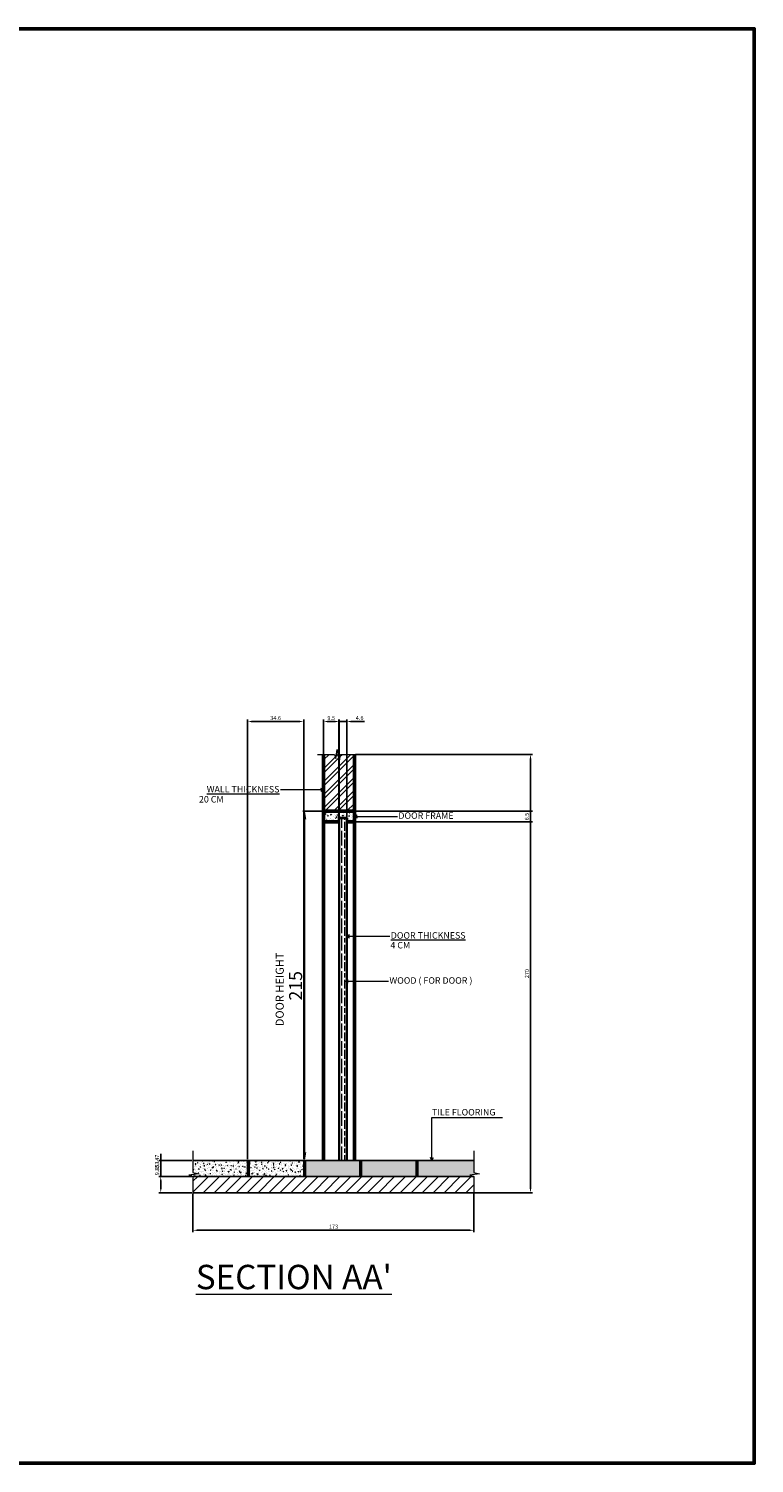
# Model space of a CAD drawing. Units: centimetres. Extents: x 1523 to 2760, y 1250 to 2134.
# Tile 4 of 4: x 2313 to 2760, y 1250 to 2134. Entities that reach past the tile are written whole.
import ezdxf

# ---------------------------------------------------------------- set-up
doc = ezdxf.new("R2010")
doc.units = ezdxf.units.CM
for name, color, linetype, lineweight in [('A-ANNO-DIMS', 2, 'Continuous', 18), ('A-ANNO-NPLT', 8, 'Continuous', 13), ('A-ANNO-SYMB', 7, 'Continuous', 18), ('A-ANNO-TEXT', 7, 'Continuous', 18), ('A-ANNO-TTLB', 7, 'Continuous', 50), ('A-DOOR', 4, 'Continuous', 35), ('A-DOOR-PATT', 251, 'Continuous', 13), ('A-FLOR', 7, 'Continuous', 25), ('A-FLOR-PATT', 251, 'Continuous', 13), ('A-WALL', 7, 'Continuous', 50), ('A-WALL-PATT', 251, 'Continuous', 13)]:
    doc.layers.add(name, color=color, linetype=linetype, lineweight=lineweight)
doc.styles.get("Standard").update_dxf_attribs({"font": 'arial.ttf'})
doc.dimstyles.new('ISO-25', dxfattribs={"dimtxt": 2.5, "dimasz": 2.5, "dimexe": 1.25, "dimexo": 0.625, "dimtad": 1, "dimtxsty": 'Standard', "dimcen": 2.5, "dimadec": 0, "dimazin": 0, "dimtfac": 1, "dimtmove": 0, "dimatfit": 3, "dimfxl": 1, "dimarcsym": 0})

# ---------------------------------------------------------------- blocks, each defined once
blk = doc.blocks.new('*D6')
at = {"layer": 'A-ANNO-DIMS', "color": 0, "lineweight": -2, "transparency": 16777216}
for p, q in [((2493.72, 1651.81), (2481.66, 1651.81)), ((2493.72, 1436.81), (2481.66, 1436.81))]:
    blk.add_line(p, q, dxfattribs=at)
at = {"layer": 'A-ANNO-DIMS', "color": 0, "lineweight": 0, "transparency": 16777216}
blk.add_line((2482.91, 1441.81), (2482.91, 1646.81), dxfattribs=at)
at = {"layer": 'A-ANNO-DIMS', "color": 0, "transparency": 16777216}
for points in [[(2482.08, 1646.81), (2483.75, 1646.81), (2482.91, 1651.81)], [(2482.08, 1441.81), (2483.75, 1441.81), (2482.91, 1436.81)]]:
    blk.add_solid(points, dxfattribs=at)
at = {"layer": 'Defpoints', "color": 0, "transparency": 16777216}
for p in [(2482.91, 1651.81), (2494.34, 1651.81), (2494.34, 1436.81)]:
    blk.add_point(p, dxfattribs=at)
at = {"layer": 'A-ANNO-DIMS', "color": 0, "transparency": 16777216, "insert": (2478.2, 1544.31), "char_height": 8, "width": 6.4304, "attachment_point": 5, "rotation": 90}
blk.add_mtext('215', dxfattribs=at)
blk = doc.blocks.new('BREAK-FLOOR')
for p, q in [((2.59, 31.69), (2.59, 18.28)), ((2.59, 18.28), (5.9, 17.46)), ((5.9, 17.46), (0, 16.6)), ((0, 16.6), (2.59, 15.97)), ((2.59, 15.97), (2.59, 0))]:
    blk.add_line(p, q)
blk = doc.blocks.new('LEADER-NOTE')
for q in [(1.66, 1.91), (26.45, 0.95), (1.66, 0)]:
    blk.add_line((0, 0.95), q)
blk = doc.blocks.new('BREAK-WALL-SECT')
for p, q in [((0, 5.33), (10.43, 5.33)), ((10.43, 5.33), (11.33, 2.85)), ((11.33, 2.85), (12, 8.33)), ((12, 8.33), (13.36, 0)), ((13.36, 0), (14.23, 5.33)), ((14.23, 5.33), (25.25, 5.33))]:
    blk.add_line(p, q)
blk = doc.blocks.new('*D28')
at = {"layer": 'A-ANNO-DIMS', "color": 0, "lineweight": -2, "transparency": 16777216}
for p, q in [((2413.97, 1416.19), (2413.97, 1392.49)), ((2586.97, 1416.19), (2586.97, 1392.49)), ((2416.47, 1393.74), (2584.47, 1393.74))]:
    blk.add_line(p, q, dxfattribs=at)
at = {"layer": 'A-ANNO-DIMS', "color": 0, "transparency": 16777216}
for points in [[(2416.47, 1394.16), (2416.47, 1393.32), (2413.97, 1393.74)], [(2584.47, 1394.16), (2584.47, 1393.32), (2586.97, 1393.74)]]:
    blk.add_solid(points, dxfattribs=at)
at = {"layer": 'Defpoints', "color": 0, "transparency": 16777216}
for p in [(2413.97, 1416.81), (2586.97, 1416.81), (2586.97, 1393.74)]:
    blk.add_point(p, dxfattribs=at)
at = {"layer": 'A-ANNO-DIMS', "color": 0, "transparency": 16777216, "insert": (2500.47, 1395.64), "char_height": 2.5, "attachment_point": 5}
blk.add_mtext('173', dxfattribs=at)
blk = doc.blocks.new('*D29')
at = {"layer": 'A-ANNO-DIMS', "color": 0, "lineweight": -2, "transparency": 16777216}
for p, q in [((2513.97, 1686.81), (2623.03, 1686.81)), ((2621.78, 1419.31), (2621.78, 1684.31)), ((2587.6, 1416.81), (2623.03, 1416.81))]:
    blk.add_line(p, q, dxfattribs=at)
at = {"layer": 'A-ANNO-DIMS', "color": 0, "transparency": 16777216}
for points in [[(2621.36, 1684.31), (2622.2, 1684.31), (2621.78, 1686.81)], [(2621.36, 1419.31), (2622.2, 1419.31), (2621.78, 1416.81)]]:
    blk.add_solid(points, dxfattribs=at)
at = {"layer": 'Defpoints', "color": 0, "transparency": 16777216}
for p in [(2513.34, 1686.81), (2621.78, 1686.81), (2586.97, 1416.81)]:
    blk.add_point(p, dxfattribs=at)
at = {"layer": 'A-ANNO-DIMS', "color": 0, "transparency": 16777216, "insert": (2619.88, 1551.81), "char_height": 2.5, "attachment_point": 5, "rotation": 90}
blk.add_mtext('270', dxfattribs=at)
blk = doc.blocks.new('*D30')
at = {"layer": 'A-ANNO-DIMS', "color": 0, "lineweight": -2, "transparency": 16777216}
for p, q in [((2513.97, 1651.81), (2623.03, 1651.81)), ((2513.97, 1645.31), (2623.03, 1645.31)), ((2621.78, 1647.81), (2621.78, 1649.31))]:
    blk.add_line(p, q, dxfattribs=at)
at = {"layer": 'A-ANNO-DIMS', "color": 0, "transparency": 16777216}
for points in [[(2621.36, 1649.31), (2622.2, 1649.31), (2621.78, 1651.81)], [(2621.36, 1647.81), (2622.2, 1647.81), (2621.78, 1645.31)]]:
    blk.add_solid(points, dxfattribs=at)
at = {"layer": 'Defpoints', "color": 0, "transparency": 16777216}
for p in [(2513.34, 1651.81), (2513.34, 1645.31), (2621.78, 1651.81)]:
    blk.add_point(p, dxfattribs=at)
at = {"layer": 'A-ANNO-DIMS', "color": 0, "transparency": 16777216, "insert": (2619.88, 1648.56), "char_height": 2.5, "attachment_point": 5, "rotation": 90}
blk.add_mtext('6.5', dxfattribs=at)
blk = doc.blocks.new('*D31')
at = {"layer": 'A-ANNO-DIMS', "color": 0, "lineweight": -2, "transparency": 16777216}
for p, q in [((2494.34, 1645.94), (2494.34, 1708.31)), ((2496.84, 1707.06), (2501.34, 1707.06)), ((2503.84, 1645.94), (2503.84, 1708.31))]:
    blk.add_line(p, q, dxfattribs=at)
at = {"layer": 'A-ANNO-DIMS', "color": 0, "transparency": 16777216}
for points in [[(2496.84, 1707.48), (2496.84, 1706.64), (2494.34, 1707.06)], [(2501.34, 1707.48), (2501.34, 1706.64), (2503.84, 1707.06)]]:
    blk.add_solid(points, dxfattribs=at)
at = {"layer": 'Defpoints', "color": 0, "transparency": 16777216}
for p in [(2503.84, 1707.06), (2494.34, 1645.31), (2503.84, 1645.31)]:
    blk.add_point(p, dxfattribs=at)
at = {"layer": 'A-ANNO-DIMS', "color": 0, "transparency": 16777216, "insert": (2499.09, 1708.96), "char_height": 2.5, "attachment_point": 5}
blk.add_mtext('9.5', dxfattribs=at)
blk = doc.blocks.new('*D32')
at = {"layer": 'A-ANNO-DIMS', "color": 0, "lineweight": -2, "transparency": 16777216}
for p, q in [((2501.54, 1707.06), (2499.04, 1707.06)), ((2504.04, 1648.24), (2504.04, 1708.31)), ((2504.04, 1707.06), (2508.64, 1707.06)), ((2508.64, 1648.24), (2508.64, 1708.31)), ((2511.14, 1707.06), (2519.54, 1707.06))]:
    blk.add_line(p, q, dxfattribs=at)
at = {"layer": 'A-ANNO-DIMS', "color": 0, "transparency": 16777216}
for points in [[(2501.54, 1707.48), (2501.54, 1706.64), (2504.04, 1707.06)], [(2511.14, 1707.48), (2511.14, 1706.64), (2508.64, 1707.06)]]:
    blk.add_solid(points, dxfattribs=at)
at = {"layer": 'Defpoints', "color": 0, "transparency": 16777216}
for p in [(2508.64, 1707.06), (2504.04, 1647.61), (2508.64, 1647.61)]:
    blk.add_point(p, dxfattribs=at)
at = {"layer": 'A-ANNO-DIMS', "color": 0, "transparency": 16777216, "insert": (2516.59, 1708.96), "char_height": 2.5, "attachment_point": 5}
blk.add_mtext('4.6', dxfattribs=at)
blk = doc.blocks.new('*D33')
at = {"layer": 'A-ANNO-DIMS', "color": 0, "lineweight": -2, "transparency": 16777216}
for p, q in [((2413.35, 1436.81), (2392.88, 1436.81)), ((2394.13, 1429.46), (2394.13, 1434.31)), ((2413.35, 1426.96), (2392.88, 1426.96))]:
    blk.add_line(p, q, dxfattribs=at)
at = {"layer": 'A-ANNO-DIMS', "color": 0, "transparency": 16777216}
for points in [[(2393.72, 1434.31), (2394.55, 1434.31), (2394.13, 1436.81)], [(2393.72, 1429.46), (2394.55, 1429.46), (2394.13, 1426.96)]]:
    blk.add_solid(points, dxfattribs=at)
at = {"layer": 'Defpoints', "color": 0, "transparency": 16777216}
for p in [(2394.13, 1436.81), (2413.97, 1436.81), (2413.98, 1426.96)]:
    blk.add_point(p, dxfattribs=at)
at = {"layer": 'A-ANNO-DIMS', "color": 0, "transparency": 16777216, "insert": (2392.23, 1431.88), "char_height": 2.5, "attachment_point": 5, "rotation": 90}
blk.add_mtext('9.853', dxfattribs=at)
blk = doc.blocks.new('*D34')
at = {"layer": 'A-ANNO-DIMS', "color": 0, "lineweight": -2, "transparency": 16777216}
for p, q in [((2394.13, 1426.96), (2394.13, 1440.85)), ((2413.35, 1426.96), (2392.88, 1426.96)), ((2394.13, 1419.31), (2394.13, 1424.46)), ((2413.35, 1416.81), (2392.88, 1416.81))]:
    blk.add_line(p, q, dxfattribs=at)
at = {"layer": 'A-ANNO-DIMS', "color": 0, "transparency": 16777216}
for points in [[(2393.72, 1424.46), (2394.55, 1424.46), (2394.13, 1426.96)], [(2393.72, 1419.31), (2394.55, 1419.31), (2394.13, 1416.81)]]:
    blk.add_solid(points, dxfattribs=at)
at = {"layer": 'Defpoints', "color": 0, "transparency": 16777216}
for p in [(2394.13, 1426.96), (2413.98, 1426.96), (2413.97, 1416.81)]:
    blk.add_point(p, dxfattribs=at)
at = {"layer": 'A-ANNO-DIMS', "color": 0, "transparency": 16777216, "insert": (2392.23, 1435.15), "char_height": 2.5, "attachment_point": 5, "rotation": 90}
blk.add_mtext('10.147', dxfattribs=at)
blk = doc.blocks.new('*D35')
at = {"layer": 'A-ANNO-DIMS', "color": 0, "lineweight": -2, "transparency": 16777216}
for p, q in [((2447.57, 1437.44), (2447.57, 1708.31)), ((2450.07, 1707.06), (2479.67, 1707.06)), ((2482.17, 1437.44), (2482.17, 1708.31))]:
    blk.add_line(p, q, dxfattribs=at)
at = {"layer": 'A-ANNO-DIMS', "color": 0, "transparency": 16777216}
for points in [[(2450.07, 1707.48), (2450.07, 1706.64), (2447.57, 1707.06)], [(2479.67, 1707.48), (2479.67, 1706.64), (2482.17, 1707.06)]]:
    blk.add_solid(points, dxfattribs=at)
at = {"layer": 'Defpoints', "color": 0, "transparency": 16777216}
for p in [(2482.17, 1707.06), (2447.57, 1436.81), (2482.17, 1436.81)]:
    blk.add_point(p, dxfattribs=at)
at = {"layer": 'A-ANNO-DIMS', "color": 0, "transparency": 16777216, "insert": (2464.87, 1708.96), "char_height": 2.5, "attachment_point": 5}
blk.add_mtext('34.6', dxfattribs=at)

msp = doc.modelspace()

# ---------------------------------------------------------------- hatches: boundary and pattern name
at = {"layer": 'A-DOOR-PATT'}
h = msp.add_hatch(dxfattribs=at)
h.set_pattern_fill('AR-CONC', color=256, scale=0.02)
h.paths.add_polyline_path([(2503.8407, 1647.8101), (2508.8407, 1647.8101), (2508.8407, 1645.3101), (2513.3407, 1645.3101), (2513.3407, 1651.8101), (2494.3407, 1651.8101), (2494.3407, 1645.3101), (2503.8407, 1645.3101)])
h = msp.add_hatch(dxfattribs=at)
h.set_pattern_fill('GOST_WOOD', color=256, scale=0.9)
h.paths.add_polyline_path([(2508.6407, 1647.6101), (2504.0407, 1647.6101), (2504.0407, 1646.8101), (2504.0407, 1436.8101), (2508.6407, 1436.8101)])
at = {"layer": 'A-FLOR-PATT'}
h = msp.add_hatch(dxfattribs=at)
h.set_pattern_fill('AR-CONC', color=256, scale=0.02)
h.paths.add_polyline_path([(2447.571, 1436.8101), (2413.9705, 1436.8101), (2413.9705, 1429.2714), (2417.2857, 1428.4479), (2411.3833, 1427.5924), (2413.9767, 1426.9567), (2413.9767, 1426.8101), (2447.571, 1426.8101)])
h = msp.add_hatch(dxfattribs=at)
h.set_pattern_fill('AR-CONC', color=256, scale=0.02)
h.paths.add_polyline_path([(2482.1715, 1436.8101), (2448.571, 1436.8101), (2448.571, 1426.8101), (2482.1715, 1426.8101)])
h = msp.add_hatch(dxfattribs=at)
h.set_pattern_fill('AR-CONC', color=256, scale=0.02)
h.paths.add_polyline_path([(2516.7721, 1436.8101), (2483.1715, 1436.8101), (2483.1715, 1426.8101), (2516.7721, 1426.8101)])
h.paths.add_polyline_path([(2551.3726, 1436.8101), (2517.7721, 1436.8101), (2517.7721, 1426.8101), (2551.3726, 1426.8101)])
h.paths.add_polyline_path([(2586.967, 1436.8101), (2552.3726, 1436.8101), (2552.3726, 1426.8101), (2586.9732, 1426.8101), (2586.9732, 1426.9567), (2584.3798, 1427.5924), (2590.2822, 1428.4479), (2586.967, 1429.2714)])
h = msp.add_hatch(dxfattribs=at)
h.set_pattern_fill('ANSI31', color=256, scale=1.5)
h.paths.add_polyline_path([(2586.9732, 1426.8101), (2413.9767, 1426.8101), (2413.9739, 1416.8101), (2586.9704, 1416.8101)])
at = {"layer": 'A-WALL-PATT'}
h = msp.add_hatch(dxfattribs=at)
h.set_pattern_fill('ANSI32', color=256, scale=0.6)
h.paths.add_polyline_path([(2513.3407, 1686.8101), (2504.8787, 1686.8101), (2504.0069, 1681.4783), (2502.6484, 1689.8089), (2501.9825, 1684.3261), (2501.0768, 1686.8101), (2494.3407, 1686.8101), (2494.3407, 1651.8101), (2513.3407, 1651.8101)])

# ---------------------------------------------------------------- linework, layer by layer
at = {"layer": 'A-ANNO-NPLT'}
for p in [(2448.571, 1426.8101), (2483.1715, 1426.8101), (2517.7721, 1426.8101), (2552.3726, 1426.8101)]:
    msp.add_point(p, dxfattribs=at)
at = {"layer": 'A-ANNO-TEXT'}
for p, q in [((2561.0871, 1436.8101), (2561.0871, 1463.2614)), ((2561.0871, 1463.2614), (2604.5295, 1463.2614)), ((2561.0871, 1436.8101), (2560.1325, 1438.4652)), ((2561.0871, 1436.8101), (2562.0416, 1438.4652))]:
    msp.add_line(p, q, dxfattribs=at)
at = {"layer": 'A-ANNO-TTLB'}
msp.add_lwpolyline([(1523.2447, 2133.8046), (2759.5532, 2133.8046), (2759.5532, 1250.2097), (1523.2447, 1250.2097)], close=True, dxfattribs=at)
at = {"layer": 'A-DOOR'}
for p, q in [((2503.8407, 1645.3101), (2503.8407, 1647.8101)), ((2503.8407, 1647.8101), (2508.8407, 1647.8101)), ((2504.0407, 1436.8101), (2504.0407, 1647.6101)), ((2504.0407, 1647.6101), (2508.6407, 1647.6101)), ((2504.0407, 1646.8101), (2504.0407, 1647.6101)), ((2508.6407, 1436.8101), (2508.6407, 1647.6101)), ((2508.6407, 1647.6101), (2508.6407, 1646.8101)), ((2508.8407, 1647.8101), (2508.8407, 1645.3101))]:
    msp.add_line(p, q, dxfattribs=at)
at = {"layer": 'A-FLOR'}
for p, q in [((2413.9705, 1436.8101), (2586.967, 1436.8101)), ((2447.571, 1426.8101), (2447.571, 1436.8101)), ((2448.571, 1426.8101), (2448.571, 1436.8101)), ((2482.1715, 1426.8101), (2482.1715, 1436.8101)), ((2483.1715, 1426.8101), (2483.1715, 1436.8101)), ((2516.7721, 1426.8101), (2516.7721, 1436.8101)), ((2517.7721, 1426.8101), (2517.7721, 1436.8101)), ((2551.3726, 1426.8101), (2551.3726, 1436.8101)), ((2552.3726, 1426.8101), (2552.3726, 1436.8101)), ((2413.9705, 1426.8101), (2586.9732, 1426.8101)), ((2413.9705, 1416.8101), (2586.9704, 1416.8101))]:
    msp.add_line(p, q, dxfattribs=at)
at = {"layer": 'A-WALL'}
for p, q in [((2494.3407, 1645.3101), (2494.3407, 1686.8101)), ((2513.3407, 1645.3101), (2513.3407, 1686.8101)), ((2494.3407, 1651.8101), (2513.3407, 1651.8101)), ((2494.3407, 1436.8101), (2494.3407, 1646.8101)), ((2494.3407, 1645.3101), (2503.8407, 1645.3101)), ((2513.3407, 1645.3101), (2508.8407, 1645.3101)), ((2513.3407, 1436.8101), (2513.3407, 1646.8101))]:
    msp.add_line(p, q, dxfattribs=at)

# ---------------------------------------------------------------- block references
at = {"layer": 'A-ANNO-SYMB'}
for name, p in [('BREAK-WALL-SECT', (2490.648, 1681.478)), ('BREAK-FLOOR', (2411.383, 1410.989)), ('BREAK-FLOOR', (2584.3795, 1410.989))]:
    msp.add_blockref(name, p, dxfattribs=at)
at = {"layer": 'A-ANNO-TEXT', "rotation": 180}
msp.add_blockref('LEADER-NOTE', (2494.3409, 1665.8819), dxfattribs=at)
at = {"layer": 'A-ANNO-TEXT'}
for p in [(2513.3405, 1647.7292), (2508.6405, 1573.9517), (2507.813, 1546.185)]:
    msp.add_blockref('LEADER-NOTE', p, dxfattribs=at)

# ---------------------------------------------------------------- texts
for s, width, insert, char_height, attachment_point in [('{\\fArial Rounded MT Bold|b0|i0|c0|p34;20 CM}', 86.463106, (2417.6635, 1661.1923), 4, 1), ('{\\fArial Rounded MT Bold|b0|i0|c0|p34;\\LWALL THICKNESS}', 86.463106, (2467.2274, 1667.3749), 4, 3), ('{\\fArial Rounded MT Bold|b0|i0|c0|p34;DOOR FRAME}', 86.463106, (2540.454, 1651.1309), 4, 1), ('{\\fArial Rounded MT Bold|b0|i0|c0|p34;\\LDOOR THICKNESS}', 86.463106, (2535.754, 1577.3535), 4, 1), ('{\\fArial Rounded MT Bold|b0|i0|c0|p34;4 CM}', 86.463106, (2535.5337, 1571.3013), 4, 1), ('{\\fArial Rounded MT Bold|b0|i0|c0|p34;WOOD ( FOR DOOR )}', 86.463106, (2534.9265, 1549.5868), 4, 1), ('{\\fArial Rounded MT Bold|b0|i0|c0|p34;TILE FLOORING}', 86.463106, (2561.1132, 1468.4454), 4, 1), ("{\\fArial Rounded MT Bold|b0|i0|c0|p34;\\LSECTION AA'}", 142.942226, (2415.7247, 1372.4557), 15, 1)]:
    msp.add_mtext_dynamic_manual_height_columns(s, width=width, gutter_width=12.5, heights=[0], dxfattribs=dict(at, insert=insert, char_height=char_height, attachment_point=attachment_point))
at = {"layer": 'A-ANNO-TEXT', "insert": (2469.8695, 1519.4169), "char_height": 5, "attachment_point": 7, "rotation": 90}
msp.add_mtext_dynamic_manual_height_columns('{\\fArial Rounded MT Bold|b0|i0|c0|p34;DOOR HEIGHT}', width=86.463106, gutter_width=12.5, heights=[0], dxfattribs=at)

# ---------------------------------------------------------------- dimensions: what is measured, and where the dimension line sits
at = {"layer": 'A-ANNO-DIMS'}
for base, p1, p2, override, picture, middle in [((2482.1715, 1707.0589), (2447.571, 1436.8101), (2482.1715, 1436.8101), {"dimdec": 1, "dimlfac": 1, "dimrnd": 0, "dimzin": 0, "dimdsep": 46, "dimlunit": 2}, '*D35', (2464.8713, 1708.9612)), ((2503.8407, 1707.0589), (2494.3407, 1645.3101), (2503.8407, 1645.3101), {"dimdec": 1, "dimlfac": 1, "dimrnd": 0, "dimzin": 0, "dimdsep": 46, "dimlunit": 2}, '*D31', (2499.0907, 1708.9603)), ((2508.6407, 1707.0589), (2504.0407, 1647.6101), (2508.6407, 1647.6101), {"dimdec": 1, "dimlfac": 1, "dimrnd": 0, "dimzin": 0, "dimdsep": 46, "dimlunit": 2}, '*D32', (2516.5909, 1708.9603)), ((2586.9704, 1393.7394), (2413.9705, 1416.8101), (2586.9704, 1416.8101), {"dimdec": 0, "dimlfac": 1, "dimrnd": 0, "dimzin": 0, "dimdsep": 46, "dimlunit": 2}, '*D28', (2500.4704, 1395.6417))]:
    dim = msp.add_linear_dim(base=base, p1=p1, p2=p2, dimstyle='ISO-25', override=override, dxfattribs=at)
    dim.commit()
    dim.dimension.update_dxf_attribs({"geometry": picture, "text_midpoint": middle})
for base, p1, p2, override, picture, middle in [((2621.7795, 1686.8101), (2586.9704, 1416.8101), (2513.3407, 1686.8101), {"dimdec": 0, "dimlfac": 1, "dimrnd": 0, "dimzin": 0, "dimdsep": 46, "dimlunit": 2}, '*D29', (2619.878, 1551.8101)), ((2482.9123, 1651.8101), (2494.3407, 1436.8101), (2494.3407, 1651.8101), {"dimtxt": 8, "dimasz": 5, "dimclrd": 0, "dimclre": 0, "dimclrt": 0, "dimlwd": 0}, '*D6', (2478.2028, 1544.3101)), ((2621.7795, 1651.8101), (2513.3407, 1645.3101), (2513.3407, 1651.8101), {"dimdec": 1, "dimlfac": 1, "dimrnd": 0, "dimzin": 0, "dimdsep": 46, "dimlunit": 2}, '*D30', (2619.878, 1648.5601)), ((2394.1333, 1426.9567), (2413.9705, 1416.8101), (2413.9767, 1426.9567), {"dimdec": 3, "dimlfac": 1, "dimrnd": 0, "dimzin": 0, "dimdsep": 46, "dimlunit": 2}, '*D34', (2392.2319, 1435.1533)), ((2394.1333, 1436.8101), (2413.9767, 1426.9567), (2413.9705, 1436.8101), {"dimdec": 3, "dimlfac": 1, "dimrnd": 0, "dimzin": 0, "dimdsep": 46, "dimlunit": 2}, '*D33', (2392.231, 1431.8834))]:
    dim = msp.add_linear_dim(base=base, p1=p1, p2=p2, angle=90, dimstyle='ISO-25', override=override, dxfattribs=at)
    dim.commit()
    dim.dimension.update_dxf_attribs({"geometry": picture, "text_midpoint": middle})

doc.saveas('drawing.dxf')
